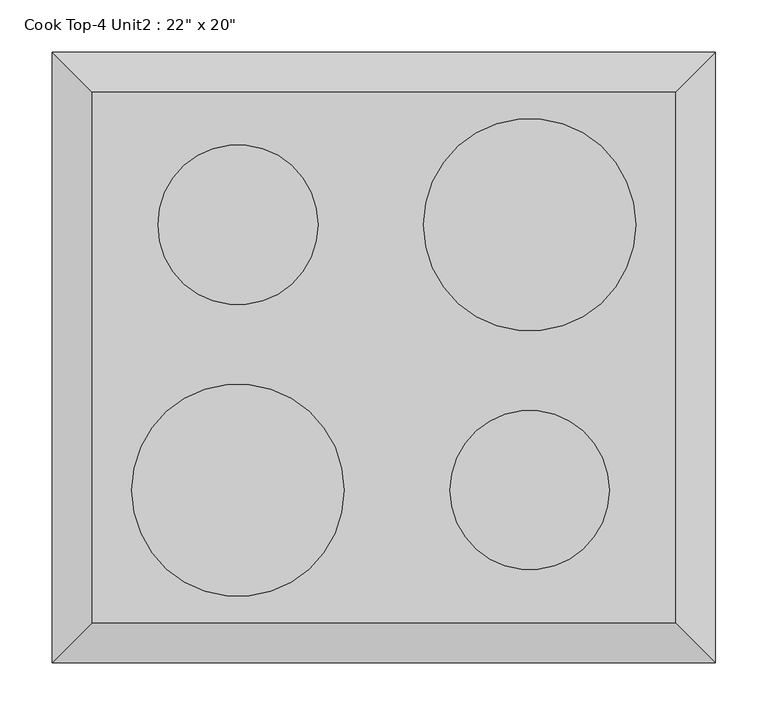
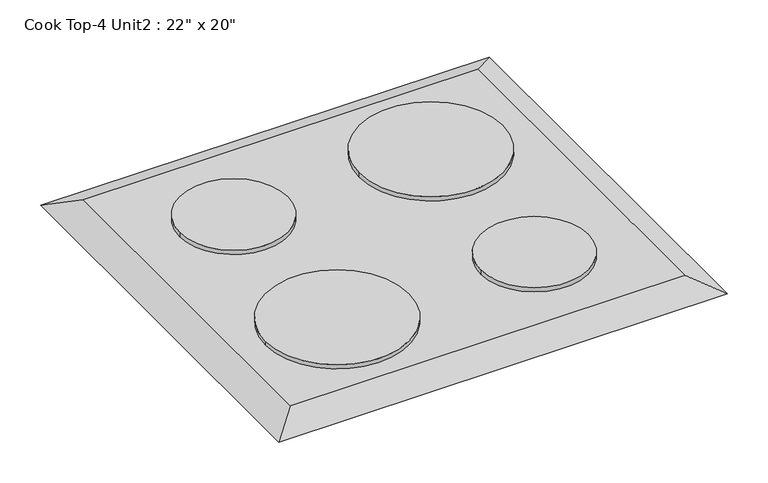
"""IFC4 building model written with IfcOpenShell, lengths in millimetres: proxy geometry."""

from ifc_helpers import new_model, si_unit, point, frame, frame_2d, origin, place, context, project, spatial, circle_curve, trimmed, segment, composite_curve, outline, extrude, faceted_brep, source, transform, mapped, element, save


def proxy_a6faaae8(model_context):
    return source(origin(), model_context, "Body", "SolidModel", [
        extrude(outline(composite_curve([segment(trimmed(circle_curve(frame_2d((-139.7, 127.0)), 76.5869489), [point((-63.1130511, 127.0))], [point((-216.2869489, 127.0))], False, "CARTESIAN"), True, "CONTINUOUS"), segment(trimmed(circle_curve(frame_2d((-139.7, 127.0)), 76.5869489), [point((-216.2869489, 127.0))], [point((-63.1130511, 127.0))], False, "CARTESIAN"), True, "CONTINUOUS")], self_intersect=False)), frame((0.0, 0.0, 918.0), z_axis=(0.0, 0.0, 1.0), x_axis=(1.0, 0.0, 0.0)), (0.0, 0.0, 1.0), 6.35),
        extrude(outline(composite_curve([segment(trimmed(circle_curve(frame_2d((139.7, -127.0)), 76.2), [point((215.9, -127.0))], [point((63.5, -127.0))], False, "CARTESIAN"), True, "CONTINUOUS"), segment(trimmed(circle_curve(frame_2d((139.7, -127.0)), 76.2), [point((63.5, -127.0))], [point((215.9, -127.0))], False, "CARTESIAN"), True, "CONTINUOUS")], self_intersect=False)), frame((0.0, 0.0, 918.0), z_axis=(0.0, 0.0, 1.0), x_axis=(1.0, 0.0, 0.0)), (0.0, 0.0, 1.0), 6.35),
        extrude(outline(composite_curve([segment(trimmed(circle_curve(frame_2d((139.7, 127.0)), 101.6), [point((38.1, 127.0))], [point((241.3, 127.0))], False, "CARTESIAN"), True, "CONTINUOUS"), segment(trimmed(circle_curve(frame_2d((139.7, 127.0)), 101.6), [point((241.3, 127.0))], [point((38.1, 127.0))], False, "CARTESIAN"), True, "CONTINUOUS")], self_intersect=False)), frame((0.0, 0.0, 918.0), z_axis=(0.0, 0.0, 1.0), x_axis=(1.0, 0.0, 0.0)), (0.0, 0.0, 1.0), 6.35),
        faceted_brep([(279.4, 254.0, 918.0), (-279.4, 254.0, 918.0), (-279.4, -254.0, 918.0), (279.4, -254.0, 918.0), (317.5, 292.1, 900.0), (317.5, -292.1, 900.0), (-317.5, -292.1, 900.0), (-317.5, 292.1, 900.0)], [[[0, 1, 2, 3]], [[4, 5, 6, 7]], [[4, 7, 1, 0]], [[7, 6, 2, 1]], [[6, 5, 3, 2]], [[5, 4, 0, 3]]]),
        extrude(outline(composite_curve([segment(trimmed(circle_curve(frame_2d((-139.7, -127.0)), 101.6), [point((-38.1, -127.0))], [point((-241.3, -127.0))], False, "CARTESIAN"), True, "CONTINUOUS"), segment(trimmed(circle_curve(frame_2d((-139.7, -127.0)), 101.6), [point((-241.3, -127.0))], [point((-38.1, -127.0))], False, "CARTESIAN"), True, "CONTINUOUS")], self_intersect=False)), frame((0.0, 0.0, 918.0), z_axis=(0.0, 0.0, 1.0), x_axis=(1.0, 0.0, 0.0)), (0.0, 0.0, 1.0), 6.35),
    ])


if __name__ == "__main__":
    model = new_model("IFC4")
    model_context = context("Model", 3, world=origin())
    ifc_project = project(units=[si_unit("LENGTHUNIT", "METRE", prefix="MILLI")], contexts=[model_context])
    site = spatial("IfcSite", under=ifc_project)
    building = spatial("IfcBuilding", under=site)
    placement = place(None, origin())
    proxy_shape = proxy_a6faaae8(model_context)
    element("IfcBuildingElementProxy", 1, Name="Cook Top-4 Unit2 : 22\" x 20\"", ObjectType="Cook Top-4 Unit2 : 22\" x 20\"", at=placement, inside=building, context=model_context, shape_type="MappedRepresentation", body=[
        mapped(proxy_shape, transform((0.0, 0.0, 0.0), x_axis=(1.0, 0.0, 0.0), y_axis=(0.0, 1.0, 0.0), z_axis=(0.0, 0.0, 1.0))),
    ])
    save(model, "model.ifc")

# Revit data of these elements
# Type "Cook Top-4 Unit2 : 22\" x 20\""
#   Depth = 1' - 8"
#   Width = 1' - 10"
#   Burner Material = Steel, Chrome Plated
#   Cooktop Material = Steel, Polished
#   Default Elevation = 0
#   Assembly Code = ""
# Element 1 (IfcBuildingElementProxy, "Cook Top-4 Unit2 : 22\" x 20\"")
#   Materials on its faces: "Steel, Chrome Plated", "Steel, Polished"
# Materials
#   "Steel, Chrome Plated": class "Metal", colour RGB 216 216 216, transparency 0, Description = "Chromiuim plated steel", Cost = 0
#   "Steel, Polished": class "Metal", colour RGB 57 57 57, transparency 0, Description = "Polished steel", Cost = 0
